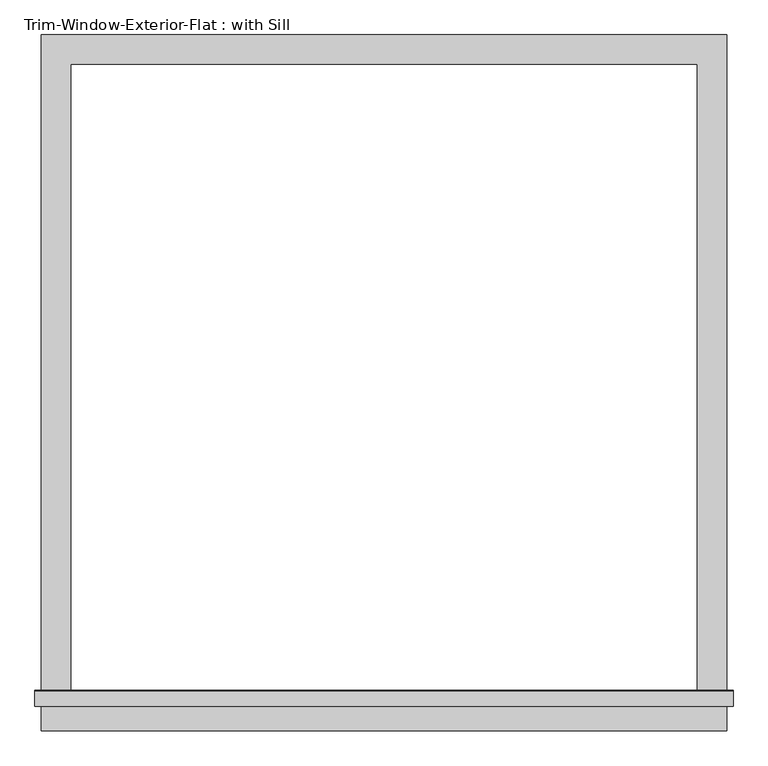
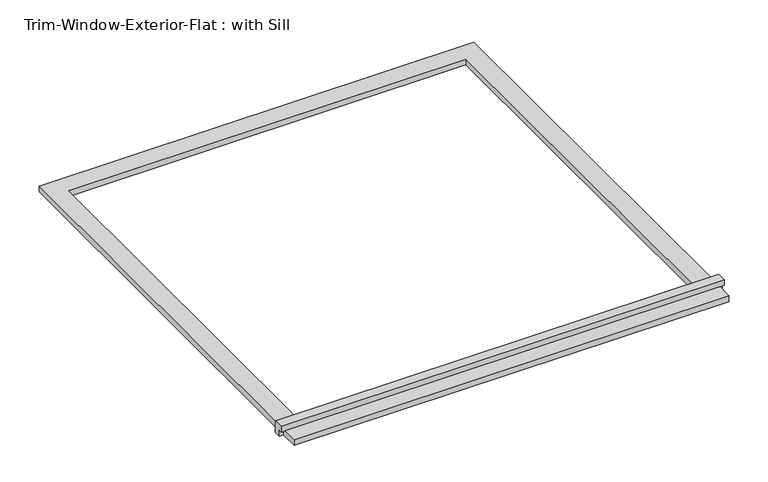
"""IFC4 building model written with IfcOpenShell, lengths in millimetres: proxy geometry, Trim-Window-Exterior-Flat : with Sill."""

from ifc_helpers import new_model, si_unit, frame, origin, origin_with_axes, place, context, project, spatial, polyline, outline, extrude, source, transform, mapped, element, save


def trim_window_exterior_flat_with_sill_7cfdd449(model_context):
    return source(origin(), model_context, "Body", "SweptSolid", [
        extrude(outline(polyline([(666.75, -1241.3823709), (666.75, -1298.5323709), (-666.75, -1298.5323709), (-666.75, -1241.3823709), (666.75, -1241.3823709)])), origin_with_axes(), (0.0, 0.0, 1.0), 19.05),
        extrude(outline(polyline([(-1250.95, 38.1), (-1221.6580645, 38.1), (-1219.2, 19.05), (-1219.2, 0.0), (-1241.3823709, 0.0), (-1241.3823709, 19.05), (-1250.95, 19.05), (-1250.95, 38.1)])), frame((-679.45, 0.0, 0.0), z_axis=(1.0, 0.0, 0.0), x_axis=(0.0, 1.0, 0.0)), (0.0, 0.0, 1.0), 1358.9),
        extrude(outline(polyline([(-666.75, 57.15), (666.75, 57.15), (666.75, -1219.2), (609.6, -1219.2), (609.6, 0.0), (-609.6, 0.0), (-609.6, -1219.2), (-666.75, -1219.2), (-666.75, 57.15)])), origin_with_axes(), (0.0, 0.0, 1.0), 19.05),
    ])


if __name__ == "__main__":
    model = new_model("IFC4")
    model_context = context("Model", 3, world=origin())
    ifc_project = project(units=[si_unit("LENGTHUNIT", "METRE", prefix="MILLI")], contexts=[model_context])
    site = spatial("IfcSite", under=ifc_project)
    building = spatial("IfcBuilding", under=site)
    placement = place(None, origin())
    trim_window_exterior_flat_with_sill_shape = trim_window_exterior_flat_with_sill_7cfdd449(model_context)
    element("IfcBuildingElementProxy", 1, Name="Trim-Window-Exterior-Flat : with Sill", ObjectType="Trim-Window-Exterior-Flat : with Sill", at=placement, inside=building, context=model_context, shape_type="MappedRepresentation", body=[
        mapped(trim_window_exterior_flat_with_sill_shape, transform((0.0, 0.0, 0.0), x_axis=(1.0, 0.0, 0.0), y_axis=(0.0, 1.0, 0.0), z_axis=(0.0, 0.0, 1.0))),
    ])
    save(model, "model.ifc")

# Revit data of these elements
# Type "Trim-Window-Exterior-Flat : with Sill"
#   Trim Width = 0' - 2 1/4"
#   Trim Thickness_Picture Frame = 0' - 1 1/4"
#   Trim Thickness_with Sill = 0' - 0 3/4"
#   Sill Thickness = 0' - 1 1/4"
#   Opening Width [instance default] = 2' - 0"
#   Opening Height [instance default] = 3' - 0"
#   Default Elevation = 4' - 0"
#   Sill = yes
#   Picture Frame = no
#   Trim Material [instance default] = none
# Element 1 (IfcBuildingElementProxy, "Trim-Window-Exterior-Flat : with Sill")
#   Opening Width = 4' - 0"
#   Opening Height = 4' - 0"
#   Trim Material = Clad - White
#   Materials on its faces: "Clad - White"
# Materials
#   "Clad - White": class "Wood", colour RGB 242 242 238, transparency 0, Cost = 0
